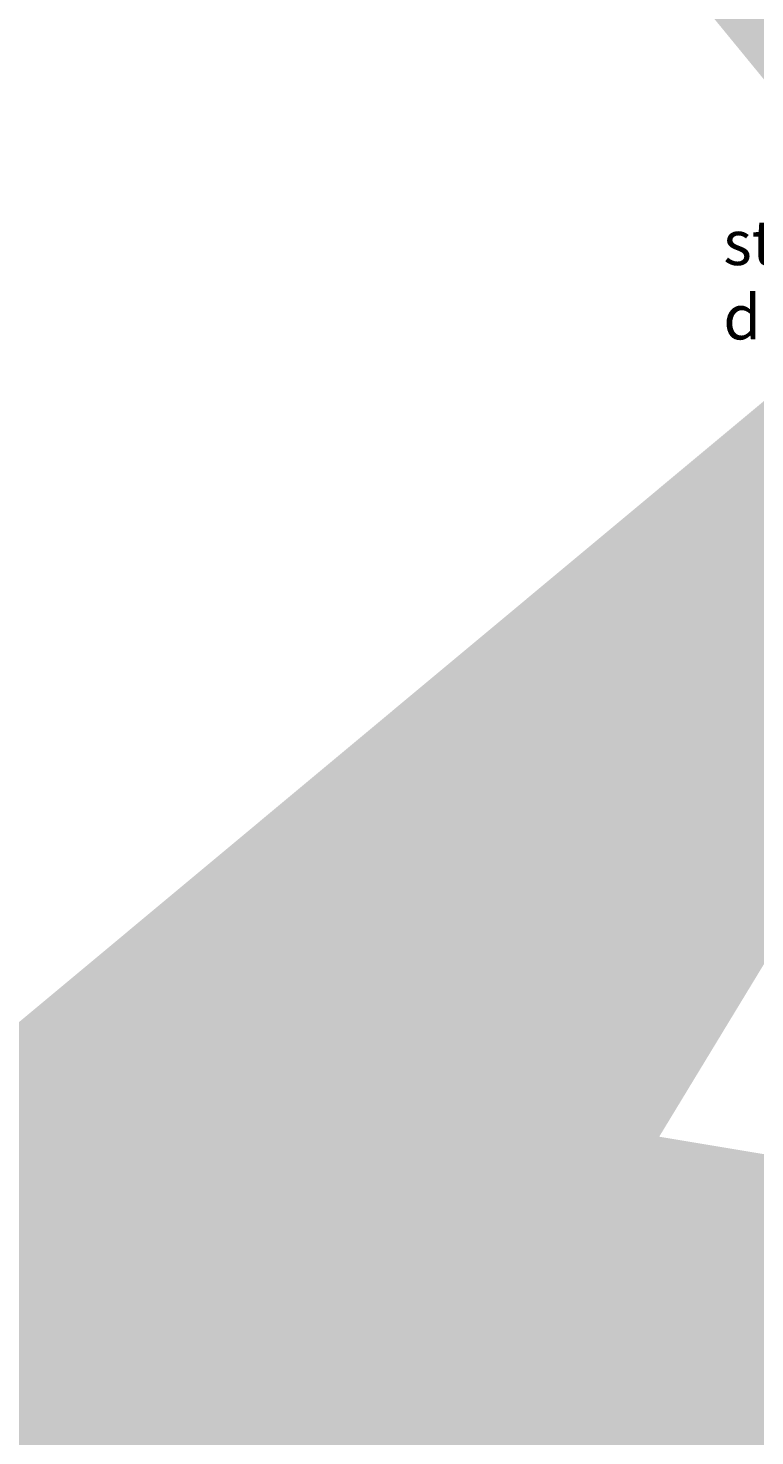
# Model space of a CAD drawing. Units: millimetres. Extents: x -22994 to 29398, y -19990 to 20176.
# Tile 8 of 135: x -44 to 5, y 5 to 99. Entities that reach past the tile are written whole.
import ezdxf

# ---------------------------------------------------------------- set-up
doc = ezdxf.new("R2010")
doc.units = ezdxf.units.MM
doc.header["$MEASUREMENT"] = 0
doc.layers.add('M-ANNO-TEXT', color=7, linetype='Continuous', lineweight=25)
doc.layers.add('M-DIMS', color=2, linetype='Continuous', lineweight=18)
doc.styles.get("Standard").update_dxf_attribs({"font": 'arial.ttf'})
doc.dimstyles.get("Standard").update_dxf_attribs({"dimtxt": 0.18, "dimasz": 10000, "dimexe": 0.18, "dimexo": 0.0625, "dimgap": 0.09, "dimtad": 0, "dimtih": 1, "dimtoh": 1, "dimdec": 0, "dimzin": 0, "dimdsep": 46, "dimtxsty": 'Standard', "dimcen": 0.09, "dimadec": 0, "dimazin": 0, "dimtfac": 1, "dimtdec": 0, "dimtofl": 0, "dimtmove": 0, "dimatfit": 3, "dimfxl": 1, "dimtolj": 1, "dimtzin": 0, "dimlwd": 30, "dimarcsym": 0})

# ---------------------------------------------------------------- blocks, each defined once
blk = doc.blocks.new('*D2')
at = {"layer": 'Defpoints', "color": 0, "transparency": 16777216}
for p in [(6.677, 10.271), (290.852, 10.271), (290.852, -5.079)]:
    blk.add_point(p, dxfattribs=at)
at = {"layer": 'M-DIMS', "color": 0, "lineweight": -2, "transparency": 16777216}
for p, q in [((6.677, 10.209), (6.677, -5.259)), ((290.852, 10.209), (290.852, -5.259))]:
    blk.add_line(p, q, dxfattribs=at)
at = {"layer": 'M-DIMS', "color": 0, "lineweight": 30, "transparency": 16777216}
for p, q in [((-9993.323, -5.079), (-19993.323, -5.079)), ((10290.852, -5.079), (20290.852, -5.079))]:
    blk.add_line(p, q, dxfattribs=at)
at = {"layer": 'M-DIMS', "color": 0, "transparency": 16777216}
for points in [[(-9993.323, 1661.588), (-9993.323, -1671.745), (6.677, -5.079)], [(10290.852, 1661.588), (10290.852, -1671.745), (290.852, -5.079)]]:
    blk.add_solid(points, dxfattribs=at)
at = {"layer": 'M-DIMS', "color": 0, "transparency": 16777216, "insert": (148.765, -5.079), "char_height": 0.18, "attachment_point": 5}
blk.add_mtext('\\A1;284.2', dxfattribs=at)
blk = doc.blocks.new('*D3')
at = {"layer": 'Defpoints', "color": 0, "transparency": 16777216}
for p in [(110.265, 204.165), (110.265, 176.366), (95.833, 127.967)]:
    blk.add_point(p, dxfattribs=at)
at = {"layer": 'M-DIMS', "color": 0, "lineweight": 30, "transparency": 16777216}
for p, q in [((-9904.167, 204.165), (-19904.167, 204.165)), ((10110.265, 204.165), (20110.265, 204.165))]:
    blk.add_line(p, q, dxfattribs=at)
at = {"layer": 'M-DIMS', "color": 0, "lineweight": -2, "transparency": 16777216}
for p, q in [((95.833, 128.03), (95.833, 204.345)), ((110.265, 176.429), (110.265, 204.345))]:
    blk.add_line(p, q, dxfattribs=at)
at = {"layer": 'M-DIMS', "color": 0, "transparency": 16777216}
for points in [[(-9904.167, 1870.832), (-9904.167, -1462.501), (95.833, 204.165)], [(10110.265, 1870.832), (10110.265, -1462.501), (110.265, 204.165)]]:
    blk.add_solid(points, dxfattribs=at)
at = {"layer": 'M-DIMS', "color": 0, "transparency": 16777216, "insert": (103.049, 204.165), "char_height": 0.18, "attachment_point": 5}
blk.add_mtext('\\A1;14.432', dxfattribs=at)
blk = doc.blocks.new('*D4')
at = {"layer": 'Defpoints', "color": 0, "transparency": 16777216}
for p in [(116.265, 204.165), (110.265, 176.366), (116.265, 176.366)]:
    blk.add_point(p, dxfattribs=at)
at = {"layer": 'M-DIMS', "color": 0, "lineweight": 30, "transparency": 16777216}
for p, q in [((-9889.735, 204.165), (-19889.735, 204.165)), ((10116.265, 204.165), (20116.265, 204.165))]:
    blk.add_line(p, q, dxfattribs=at)
at = {"layer": 'M-DIMS', "color": 0, "lineweight": -2, "transparency": 16777216}
for p, q in [((110.265, 176.429), (110.265, 204.345)), ((116.265, 176.429), (116.265, 204.345))]:
    blk.add_line(p, q, dxfattribs=at)
at = {"layer": 'M-DIMS', "color": 0, "transparency": 16777216}
for points in [[(-9889.735, 1870.832), (-9889.735, -1462.501), (110.265, 204.165)], [(10116.265, 1870.832), (10116.265, -1462.501), (116.265, 204.165)]]:
    blk.add_solid(points, dxfattribs=at)
at = {"layer": 'M-DIMS', "color": 0, "transparency": 16777216, "insert": (113.265, 204.165), "char_height": 0.18, "attachment_point": 5}
blk.add_mtext('\\A1;6', dxfattribs=at)
blk = doc.blocks.new('*D5')
at = {"layer": 'Defpoints', "color": 0, "transparency": 16777216}
for p in [(181.265, 204.165), (116.265, 176.366), (181.265, 176.366)]:
    blk.add_point(p, dxfattribs=at)
at = {"layer": 'M-DIMS', "color": 0, "lineweight": 30, "transparency": 16777216}
for p, q in [((-9883.735, 204.165), (-19883.735, 204.165)), ((10181.265, 204.165), (20181.265, 204.165))]:
    blk.add_line(p, q, dxfattribs=at)
at = {"layer": 'M-DIMS', "color": 0, "lineweight": -2, "transparency": 16777216}
for p, q in [((116.265, 176.429), (116.265, 204.345)), ((181.265, 176.429), (181.265, 204.345))]:
    blk.add_line(p, q, dxfattribs=at)
at = {"layer": 'M-DIMS', "color": 0, "transparency": 16777216}
for points in [[(-9883.735, 1870.832), (-9883.735, -1462.501), (116.265, 204.165)], [(10181.265, 1870.832), (10181.265, -1462.501), (181.265, 204.165)]]:
    blk.add_solid(points, dxfattribs=at)
at = {"layer": 'M-DIMS', "color": 0, "transparency": 16777216, "insert": (148.765, 204.165), "char_height": 0.18, "attachment_point": 5}
blk.add_mtext('\\A1;65', dxfattribs=at)
blk = doc.blocks.new('*D6')
at = {"layer": 'Defpoints', "color": 0, "transparency": 16777216}
for p in [(187.265, 204.165), (181.265, 176.366), (187.265, 176.366)]:
    blk.add_point(p, dxfattribs=at)
at = {"layer": 'M-DIMS', "color": 0, "lineweight": 30, "transparency": 16777216}
for p, q in [((-9818.735, 204.165), (-19818.735, 204.165)), ((10187.265, 204.165), (20187.265, 204.165))]:
    blk.add_line(p, q, dxfattribs=at)
at = {"layer": 'M-DIMS', "color": 0, "lineweight": -2, "transparency": 16777216}
for p, q in [((181.265, 176.429), (181.265, 204.345)), ((187.265, 176.429), (187.265, 204.345))]:
    blk.add_line(p, q, dxfattribs=at)
at = {"layer": 'M-DIMS', "color": 0, "transparency": 16777216}
for points in [[(-9818.735, 1870.832), (-9818.735, -1462.501), (181.265, 204.165)], [(10187.265, 1870.832), (10187.265, -1462.501), (187.265, 204.165)]]:
    blk.add_solid(points, dxfattribs=at)
at = {"layer": 'M-DIMS', "color": 0, "transparency": 16777216, "insert": (184.265, 204.165), "char_height": 0.18, "attachment_point": 5}
blk.add_mtext('\\A1;6', dxfattribs=at)
blk = doc.blocks.new('*D7')
at = {"layer": 'Defpoints', "color": 0, "transparency": 16777216}
for p in [(201.697, 204.165), (187.265, 176.366), (201.697, 127.967)]:
    blk.add_point(p, dxfattribs=at)
at = {"layer": 'M-DIMS', "color": 0, "lineweight": 30, "transparency": 16777216}
for p, q in [((-9812.735, 204.165), (-19812.735, 204.165)), ((10201.697, 204.165), (20201.697, 204.165))]:
    blk.add_line(p, q, dxfattribs=at)
at = {"layer": 'M-DIMS', "color": 0, "lineweight": -2, "transparency": 16777216}
for p, q in [((187.265, 176.429), (187.265, 204.345)), ((201.697, 128.03), (201.697, 204.345))]:
    blk.add_line(p, q, dxfattribs=at)
at = {"layer": 'M-DIMS', "color": 0, "transparency": 16777216}
for points in [[(-9812.735, 1870.832), (-9812.735, -1462.501), (187.265, 204.165)], [(10201.697, 1870.832), (10201.697, -1462.501), (201.697, 204.165)]]:
    blk.add_solid(points, dxfattribs=at)
at = {"layer": 'M-DIMS', "color": 0, "transparency": 16777216, "insert": (194.481, 204.165), "char_height": 0.18, "attachment_point": 5}
blk.add_mtext('\\A1;14.432', dxfattribs=at)
blk = doc.blocks.new('*D8')
at = {"layer": 'Defpoints', "color": 0, "transparency": 16777216}
for p in [(227.648, 204.165), (227.648, 146.73), (201.697, 127.967)]:
    blk.add_point(p, dxfattribs=at)
at = {"layer": 'M-DIMS', "color": 0, "lineweight": 30, "transparency": 16777216}
for p, q in [((-9798.303, 204.165), (-19798.303, 204.165)), ((10227.648, 204.165), (20227.648, 204.165))]:
    blk.add_line(p, q, dxfattribs=at)
at = {"layer": 'M-DIMS', "color": 0, "lineweight": -2, "transparency": 16777216}
for p, q in [((201.697, 128.03), (201.697, 204.345)), ((227.648, 146.792), (227.648, 204.345))]:
    blk.add_line(p, q, dxfattribs=at)
at = {"layer": 'M-DIMS', "color": 0, "transparency": 16777216}
for points in [[(-9798.303, 1870.832), (-9798.303, -1462.501), (201.697, 204.165)], [(10227.648, 1870.832), (10227.648, -1462.501), (227.648, 204.165)]]:
    blk.add_solid(points, dxfattribs=at)
at = {"layer": 'M-DIMS', "color": 0, "transparency": 16777216, "insert": (214.673, 204.165), "char_height": 0.18, "attachment_point": 5}
blk.add_mtext('\\A1;25.95', dxfattribs=at)
blk = doc.blocks.new('*D9')
at = {"layer": 'Defpoints', "color": 0, "transparency": 16777216}
for p in [(187.265, 176.366), (306.202, 176.366), (290.852, 10.271)]:
    blk.add_point(p, dxfattribs=at)
at = {"layer": 'M-DIMS', "color": 0, "lineweight": 30, "transparency": 16777216}
for p, q in [((306.202, 10176.366), (306.202, 20176.366)), ((306.202, -9989.729), (306.202, -19989.729))]:
    blk.add_line(p, q, dxfattribs=at)
at = {"layer": 'M-DIMS', "color": 0, "lineweight": -2, "transparency": 16777216}
for p, q in [((187.327, 176.366), (306.382, 176.366)), ((290.915, 10.271), (306.382, 10.271))]:
    blk.add_line(p, q, dxfattribs=at)
at = {"layer": 'M-DIMS', "color": 0, "transparency": 16777216}
for points in [[(-1360.465, 10176.366), (1972.869, 10176.366), (306.202, 176.366)], [(-1360.465, -9989.729), (1972.869, -9989.729), (306.202, 10.271)]]:
    blk.add_solid(points, dxfattribs=at)
at = {"layer": 'M-DIMS', "color": 0, "transparency": 16777216, "insert": (306.202, 93.319), "char_height": 0.18, "attachment_point": 5}
blk.add_mtext('\\A1;166.1', dxfattribs=at)
blk = doc.blocks.new('*D10')
at = {"layer": 'Defpoints', "color": 0, "transparency": 16777216}
for p in [(125.65, 136.071), (133.346, 136.071), (133.346, -5.079)]:
    blk.add_point(p, dxfattribs=at)
at = {"layer": 'M-DIMS', "color": 0, "lineweight": -2, "transparency": 16777216}
for p, q in [((125.65, 136.009), (125.65, -5.259)), ((133.346, 136.009), (133.346, -5.259))]:
    blk.add_line(p, q, dxfattribs=at)
at = {"layer": 'M-DIMS', "color": 0, "lineweight": 30, "transparency": 16777216}
for p, q in [((-9874.35, -5.079), (-19874.35, -5.079)), ((10133.346, -5.079), (20133.346, -5.079))]:
    blk.add_line(p, q, dxfattribs=at)
at = {"layer": 'M-DIMS', "color": 0, "transparency": 16777216}
for points in [[(-9874.35, 1661.588), (-9874.35, -1671.745), (125.65, -5.079)], [(10133.346, 1661.588), (10133.346, -1671.745), (133.346, -5.079)]]:
    blk.add_solid(points, dxfattribs=at)
at = {"layer": 'M-DIMS', "color": 0, "transparency": 16777216, "insert": (129.498, -5.079), "char_height": 0.18, "attachment_point": 5}
blk.add_mtext('\\A1;7.696', dxfattribs=at)
blk = doc.blocks.new('*D11')
at = {"layer": 'Defpoints', "color": 0, "transparency": 16777216}
for p in [(133.346, 136.071), (135.65, 136.071), (135.65, -5.079)]:
    blk.add_point(p, dxfattribs=at)
at = {"layer": 'M-DIMS', "color": 0, "lineweight": -2, "transparency": 16777216}
for p, q in [((133.346, 136.009), (133.346, -5.259)), ((135.65, 136.009), (135.65, -5.259))]:
    blk.add_line(p, q, dxfattribs=at)
at = {"layer": 'M-DIMS', "color": 0, "lineweight": 30, "transparency": 16777216}
for p, q in [((-9866.654, -5.079), (-19866.654, -5.079)), ((10135.65, -5.079), (20135.65, -5.079))]:
    blk.add_line(p, q, dxfattribs=at)
at = {"layer": 'M-DIMS', "color": 0, "transparency": 16777216}
for points in [[(-9866.654, 1661.588), (-9866.654, -1671.745), (133.346, -5.079)], [(10135.65, 1661.588), (10135.65, -1671.745), (135.65, -5.079)]]:
    blk.add_solid(points, dxfattribs=at)
at = {"layer": 'M-DIMS', "color": 0, "transparency": 16777216, "insert": (134.498, -5.079), "char_height": 0.18, "attachment_point": 5}
blk.add_mtext('\\A1;2.304', dxfattribs=at)
blk = doc.blocks.new('*D12')
at = {"layer": 'Defpoints', "color": 0, "transparency": 16777216}
for p in [(135.65, 136.071), (145.65, 136.071), (145.65, -5.079)]:
    blk.add_point(p, dxfattribs=at)
at = {"layer": 'M-DIMS', "color": 0, "lineweight": -2, "transparency": 16777216}
for p, q in [((135.65, 136.009), (135.65, -5.259)), ((145.65, 136.009), (145.65, -5.259))]:
    blk.add_line(p, q, dxfattribs=at)
at = {"layer": 'M-DIMS', "color": 0, "lineweight": 30, "transparency": 16777216}
for p, q in [((-9864.35, -5.079), (-19864.35, -5.079)), ((10145.65, -5.079), (20145.65, -5.079))]:
    blk.add_line(p, q, dxfattribs=at)
at = {"layer": 'M-DIMS', "color": 0, "transparency": 16777216}
for points in [[(-9864.35, 1661.588), (-9864.35, -1671.745), (135.65, -5.079)], [(10145.65, 1661.588), (10145.65, -1671.745), (145.65, -5.079)]]:
    blk.add_solid(points, dxfattribs=at)
at = {"layer": 'M-DIMS', "color": 0, "transparency": 16777216, "insert": (140.65, -5.079), "char_height": 0.18, "attachment_point": 5}
blk.add_mtext('\\A1;10', dxfattribs=at)
blk = doc.blocks.new('*D13')
at = {"layer": 'Defpoints', "color": 0, "transparency": 16777216}
for p in [(145.65, 136.071), (155.65, 136.071), (155.65, -5.079)]:
    blk.add_point(p, dxfattribs=at)
at = {"layer": 'M-DIMS', "color": 0, "lineweight": -2, "transparency": 16777216}
for p, q in [((145.65, 136.009), (145.65, -5.259)), ((155.65, 136.009), (155.65, -5.259))]:
    blk.add_line(p, q, dxfattribs=at)
at = {"layer": 'M-DIMS', "color": 0, "lineweight": 30, "transparency": 16777216}
for p, q in [((-9854.35, -5.079), (-19854.35, -5.079)), ((10155.65, -5.079), (20155.65, -5.079))]:
    blk.add_line(p, q, dxfattribs=at)
at = {"layer": 'M-DIMS', "color": 0, "transparency": 16777216}
for points in [[(-9854.35, 1661.588), (-9854.35, -1671.745), (145.65, -5.079)], [(10155.65, 1661.588), (10155.65, -1671.745), (155.65, -5.079)]]:
    blk.add_solid(points, dxfattribs=at)
at = {"layer": 'M-DIMS', "color": 0, "transparency": 16777216, "insert": (150.65, -5.079), "char_height": 0.18, "attachment_point": 5}
blk.add_mtext('\\A1;10', dxfattribs=at)
blk = doc.blocks.new('*D14')
at = {"layer": 'Defpoints', "color": 0, "transparency": 16777216}
for p in [(155.65, 136.071), (165.65, 136.071), (165.65, -5.079)]:
    blk.add_point(p, dxfattribs=at)
at = {"layer": 'M-DIMS', "color": 0, "lineweight": -2, "transparency": 16777216}
for p, q in [((155.65, 136.009), (155.65, -5.259)), ((165.65, 136.009), (165.65, -5.259))]:
    blk.add_line(p, q, dxfattribs=at)
at = {"layer": 'M-DIMS', "color": 0, "lineweight": 30, "transparency": 16777216}
for p, q in [((-9844.35, -5.079), (-19844.35, -5.079)), ((10165.65, -5.079), (20165.65, -5.079))]:
    blk.add_line(p, q, dxfattribs=at)
at = {"layer": 'M-DIMS', "color": 0, "transparency": 16777216}
for points in [[(-9844.35, 1661.588), (-9844.35, -1671.745), (155.65, -5.079)], [(10165.65, 1661.588), (10165.65, -1671.745), (165.65, -5.079)]]:
    blk.add_solid(points, dxfattribs=at)
at = {"layer": 'M-DIMS', "color": 0, "transparency": 16777216, "insert": (160.65, -5.079), "char_height": 0.18, "attachment_point": 5}
blk.add_mtext('\\A1;10', dxfattribs=at)
blk = doc.blocks.new('*D15')
at = {"layer": 'Defpoints', "color": 0, "transparency": 16777216}
for p in [(173.346, 154.788), (173.346, 136.071), (306.202, 136.071)]:
    blk.add_point(p, dxfattribs=at)
at = {"layer": 'M-DIMS', "color": 0, "lineweight": 30, "transparency": 16777216}
for p, q in [((306.202, 10154.788), (306.202, 20154.788)), ((306.202, -9863.929), (306.202, -19863.929))]:
    blk.add_line(p, q, dxfattribs=at)
at = {"layer": 'M-DIMS', "color": 0, "lineweight": -2, "transparency": 16777216}
for p, q in [((173.408, 154.788), (306.382, 154.788)), ((173.408, 136.071), (306.382, 136.071))]:
    blk.add_line(p, q, dxfattribs=at)
at = {"layer": 'M-DIMS', "color": 0, "transparency": 16777216}
for points in [[(-1360.465, 10154.788), (1972.869, 10154.788), (306.202, 154.788)], [(-1360.465, -9863.929), (1972.869, -9863.929), (306.202, 136.071)]]:
    blk.add_solid(points, dxfattribs=at)
at = {"layer": 'M-DIMS', "color": 0, "transparency": 16777216, "insert": (306.202, 145.43), "char_height": 0.18, "attachment_point": 5}
blk.add_mtext('\\A1;18.717', dxfattribs=at)
blk = doc.blocks.new('*D16')
at = {"layer": 'Defpoints', "color": 0, "transparency": 16777216}
for p in [(120.17, 204.165), (110.466, 48.035), (120.17, 48.035)]:
    blk.add_point(p, dxfattribs=at)
at = {"layer": 'M-DIMS', "color": 0, "lineweight": 30, "transparency": 16777216}
for p, q in [((-9889.534, 204.165), (-19889.534, 204.165)), ((10120.17, 204.165), (20120.17, 204.165))]:
    blk.add_line(p, q, dxfattribs=at)
at = {"layer": 'M-DIMS', "color": 0, "lineweight": -2, "transparency": 16777216}
for p, q in [((110.466, 48.097), (110.466, 204.345)), ((120.17, 48.097), (120.17, 204.345))]:
    blk.add_line(p, q, dxfattribs=at)
at = {"layer": 'M-DIMS', "color": 0, "transparency": 16777216}
for points in [[(-9889.534, 1870.832), (-9889.534, -1462.501), (110.466, 204.165)], [(10120.17, 1870.832), (10120.17, -1462.501), (120.17, 204.165)]]:
    blk.add_solid(points, dxfattribs=at)
at = {"layer": 'M-DIMS', "color": 0, "transparency": 16777216, "insert": (115.318, 204.165), "char_height": 0.18, "attachment_point": 5}
blk.add_mtext('\\A1;9.704', dxfattribs=at)
blk = doc.blocks.new('*D17')
at = {"layer": 'Defpoints', "color": 0, "transparency": 16777216}
for p in [(126.17, 204.165), (120.17, 48.035), (126.17, 48.035)]:
    blk.add_point(p, dxfattribs=at)
at = {"layer": 'M-DIMS', "color": 0, "lineweight": 30, "transparency": 16777216}
for p, q in [((-9879.83, 204.165), (-19879.83, 204.165)), ((10126.17, 204.165), (20126.17, 204.165))]:
    blk.add_line(p, q, dxfattribs=at)
at = {"layer": 'M-DIMS', "color": 0, "lineweight": -2, "transparency": 16777216}
for p, q in [((120.17, 48.097), (120.17, 204.345)), ((126.17, 48.097), (126.17, 204.345))]:
    blk.add_line(p, q, dxfattribs=at)
at = {"layer": 'M-DIMS', "color": 0, "transparency": 16777216}
for points in [[(-9879.83, 1870.832), (-9879.83, -1462.501), (120.17, 204.165)], [(10126.17, 1870.832), (10126.17, -1462.501), (126.17, 204.165)]]:
    blk.add_solid(points, dxfattribs=at)
at = {"layer": 'M-DIMS', "color": 0, "transparency": 16777216, "insert": (123.17, 204.165), "char_height": 0.18, "attachment_point": 5}
blk.add_mtext('\\A1;6', dxfattribs=at)
blk = doc.blocks.new('*D18')
at = {"layer": 'Defpoints', "color": 0, "transparency": 16777216}
for p in [(132.17, 204.165), (126.17, 48.035), (132.17, 48.035)]:
    blk.add_point(p, dxfattribs=at)
at = {"layer": 'M-DIMS', "color": 0, "lineweight": 30, "transparency": 16777216}
for p, q in [((-9873.83, 204.165), (-19873.83, 204.165)), ((10132.17, 204.165), (20132.17, 204.165))]:
    blk.add_line(p, q, dxfattribs=at)
at = {"layer": 'M-DIMS', "color": 0, "lineweight": -2, "transparency": 16777216}
for p, q in [((126.17, 48.097), (126.17, 204.345)), ((132.17, 48.097), (132.17, 204.345))]:
    blk.add_line(p, q, dxfattribs=at)
at = {"layer": 'M-DIMS', "color": 0, "transparency": 16777216}
for points in [[(-9873.83, 1870.832), (-9873.83, -1462.501), (126.17, 204.165)], [(10132.17, 1870.832), (10132.17, -1462.501), (132.17, 204.165)]]:
    blk.add_solid(points, dxfattribs=at)
at = {"layer": 'M-DIMS', "color": 0, "transparency": 16777216, "insert": (129.17, 204.165), "char_height": 0.18, "attachment_point": 5}
blk.add_mtext('\\A1;6', dxfattribs=at)
blk = doc.blocks.new('*D19')
at = {"layer": 'Defpoints', "color": 0, "transparency": 16777216}
for p in [(138.17, 204.165), (132.17, 48.035), (138.17, 48.035)]:
    blk.add_point(p, dxfattribs=at)
at = {"layer": 'M-DIMS', "color": 0, "lineweight": 30, "transparency": 16777216}
for p, q in [((-9867.83, 204.165), (-19867.83, 204.165)), ((10138.17, 204.165), (20138.17, 204.165))]:
    blk.add_line(p, q, dxfattribs=at)
at = {"layer": 'M-DIMS', "color": 0, "lineweight": -2, "transparency": 16777216}
for p, q in [((132.17, 48.097), (132.17, 204.345)), ((138.17, 48.097), (138.17, 204.345))]:
    blk.add_line(p, q, dxfattribs=at)
at = {"layer": 'M-DIMS', "color": 0, "transparency": 16777216}
for points in [[(-9867.83, 1870.832), (-9867.83, -1462.501), (132.17, 204.165)], [(10138.17, 1870.832), (10138.17, -1462.501), (138.17, 204.165)]]:
    blk.add_solid(points, dxfattribs=at)
at = {"layer": 'M-DIMS', "color": 0, "transparency": 16777216, "insert": (135.17, 204.165), "char_height": 0.18, "attachment_point": 5}
blk.add_mtext('\\A1;6', dxfattribs=at)
blk = doc.blocks.new('*D20')
at = {"layer": 'Defpoints', "color": 0, "transparency": 16777216}
for p in [(144.17, 204.165), (138.17, 48.035), (144.17, 48.035)]:
    blk.add_point(p, dxfattribs=at)
at = {"layer": 'M-DIMS', "color": 0, "lineweight": 30, "transparency": 16777216}
for p, q in [((-9861.83, 204.165), (-19861.83, 204.165)), ((10144.17, 204.165), (20144.17, 204.165))]:
    blk.add_line(p, q, dxfattribs=at)
at = {"layer": 'M-DIMS', "color": 0, "lineweight": -2, "transparency": 16777216}
for p, q in [((138.17, 48.097), (138.17, 204.345)), ((144.17, 48.097), (144.17, 204.345))]:
    blk.add_line(p, q, dxfattribs=at)
at = {"layer": 'M-DIMS', "color": 0, "transparency": 16777216}
for points in [[(-9861.83, 1870.832), (-9861.83, -1462.501), (138.17, 204.165)], [(10144.17, 1870.832), (10144.17, -1462.501), (144.17, 204.165)]]:
    blk.add_solid(points, dxfattribs=at)
at = {"layer": 'M-DIMS', "color": 0, "transparency": 16777216, "insert": (141.17, 204.165), "char_height": 0.18, "attachment_point": 5}
blk.add_mtext('\\A1;6', dxfattribs=at)
blk = doc.blocks.new('*D21')
at = {"layer": 'Defpoints', "color": 0, "transparency": 16777216}
for p in [(149.116, 204.165), (144.17, 48.035), (149.116, 48.035)]:
    blk.add_point(p, dxfattribs=at)
at = {"layer": 'M-DIMS', "color": 0, "lineweight": 30, "transparency": 16777216}
for p, q in [((-9855.83, 204.165), (-19855.83, 204.165)), ((10149.116, 204.165), (20149.116, 204.165))]:
    blk.add_line(p, q, dxfattribs=at)
at = {"layer": 'M-DIMS', "color": 0, "lineweight": -2, "transparency": 16777216}
for p, q in [((144.17, 48.097), (144.17, 204.345)), ((149.116, 48.097), (149.116, 204.345))]:
    blk.add_line(p, q, dxfattribs=at)
at = {"layer": 'M-DIMS', "color": 0, "transparency": 16777216}
for points in [[(-9855.83, 1870.832), (-9855.83, -1462.501), (144.17, 204.165)], [(10149.116, 1870.832), (10149.116, -1462.501), (149.116, 204.165)]]:
    blk.add_solid(points, dxfattribs=at)
at = {"layer": 'M-DIMS', "color": 0, "transparency": 16777216, "insert": (146.643, 204.165), "char_height": 0.18, "attachment_point": 5}
blk.add_mtext('\\A1;4.945', dxfattribs=at)
blk = doc.blocks.new('*D22')
at = {"layer": 'Defpoints', "color": 0, "transparency": 16777216}
for p in [(149.116, 30.99), (155.116, 30.99), (155.116, -5.079)]:
    blk.add_point(p, dxfattribs=at)
at = {"layer": 'M-DIMS', "color": 0, "lineweight": -2, "transparency": 16777216}
for p, q in [((149.116, 30.927), (149.116, -5.259)), ((155.116, 30.927), (155.116, -5.259))]:
    blk.add_line(p, q, dxfattribs=at)
at = {"layer": 'M-DIMS', "color": 0, "lineweight": 30, "transparency": 16777216}
for p, q in [((-9850.884, -5.079), (-19850.884, -5.079)), ((10155.116, -5.079), (20155.116, -5.079))]:
    blk.add_line(p, q, dxfattribs=at)
at = {"layer": 'M-DIMS', "color": 0, "transparency": 16777216}
for points in [[(-9850.884, 1661.588), (-9850.884, -1671.745), (149.116, -5.079)], [(10155.116, 1661.588), (10155.116, -1671.745), (155.116, -5.079)]]:
    blk.add_solid(points, dxfattribs=at)
at = {"layer": 'M-DIMS', "color": 0, "transparency": 16777216, "insert": (152.116, -5.079), "char_height": 0.18, "attachment_point": 5}
blk.add_mtext('\\A1;6', dxfattribs=at)
blk = doc.blocks.new('*D23')
at = {"layer": 'Defpoints', "color": 0, "transparency": 16777216}
for p in [(155.116, 30.99), (161.116, 30.99), (161.116, -5.079)]:
    blk.add_point(p, dxfattribs=at)
at = {"layer": 'M-DIMS', "color": 0, "lineweight": -2, "transparency": 16777216}
for p, q in [((155.116, 30.927), (155.116, -5.259)), ((161.116, 30.927), (161.116, -5.259))]:
    blk.add_line(p, q, dxfattribs=at)
at = {"layer": 'M-DIMS', "color": 0, "lineweight": 30, "transparency": 16777216}
for p, q in [((-9844.884, -5.079), (-19844.884, -5.079)), ((10161.116, -5.079), (20161.116, -5.079))]:
    blk.add_line(p, q, dxfattribs=at)
at = {"layer": 'M-DIMS', "color": 0, "transparency": 16777216}
for points in [[(-9844.884, 1661.588), (-9844.884, -1671.745), (155.116, -5.079)], [(10161.116, 1661.588), (10161.116, -1671.745), (161.116, -5.079)]]:
    blk.add_solid(points, dxfattribs=at)
at = {"layer": 'M-DIMS', "color": 0, "transparency": 16777216, "insert": (158.116, -5.079), "char_height": 0.18, "attachment_point": 5}
blk.add_mtext('\\A1;6', dxfattribs=at)
blk = doc.blocks.new('*D24')
at = {"layer": 'Defpoints', "color": 0, "transparency": 16777216}
for p in [(161.116, 30.99), (166.439, 30.99), (166.439, -5.079)]:
    blk.add_point(p, dxfattribs=at)
at = {"layer": 'M-DIMS', "color": 0, "lineweight": -2, "transparency": 16777216}
for p, q in [((161.116, 30.927), (161.116, -5.259)), ((166.439, 30.927), (166.439, -5.259))]:
    blk.add_line(p, q, dxfattribs=at)
at = {"layer": 'M-DIMS', "color": 0, "lineweight": 30, "transparency": 16777216}
for p, q in [((-9838.884, -5.079), (-19838.884, -5.079)), ((10166.439, -5.079), (20166.439, -5.079))]:
    blk.add_line(p, q, dxfattribs=at)
at = {"layer": 'M-DIMS', "color": 0, "transparency": 16777216}
for points in [[(-9838.884, 1661.588), (-9838.884, -1671.745), (161.116, -5.079)], [(10166.439, 1661.588), (10166.439, -1671.745), (166.439, -5.079)]]:
    blk.add_solid(points, dxfattribs=at)
at = {"layer": 'M-DIMS', "color": 0, "transparency": 16777216, "insert": (163.777, -5.079), "char_height": 0.18, "attachment_point": 5}
blk.add_mtext('\\A1;5.323', dxfattribs=at)
blk = doc.blocks.new('*D25')
at = {"layer": 'Defpoints', "color": 0, "transparency": 16777216}
for p in [(166.439, 30.99), (172.439, 30.99), (172.439, -5.079)]:
    blk.add_point(p, dxfattribs=at)
at = {"layer": 'M-DIMS', "color": 0, "lineweight": -2, "transparency": 16777216}
for p, q in [((166.439, 30.927), (166.439, -5.259)), ((172.439, 30.927), (172.439, -5.259))]:
    blk.add_line(p, q, dxfattribs=at)
at = {"layer": 'M-DIMS', "color": 0, "lineweight": 30, "transparency": 16777216}
for p, q in [((-9833.561, -5.079), (-19833.561, -5.079)), ((10172.439, -5.079), (20172.439, -5.079))]:
    blk.add_line(p, q, dxfattribs=at)
at = {"layer": 'M-DIMS', "color": 0, "transparency": 16777216}
for points in [[(-9833.561, 1661.588), (-9833.561, -1671.745), (166.439, -5.079)], [(10172.439, 1661.588), (10172.439, -1671.745), (172.439, -5.079)]]:
    blk.add_solid(points, dxfattribs=at)
at = {"layer": 'M-DIMS', "color": 0, "transparency": 16777216, "insert": (169.439, -5.079), "char_height": 0.18, "attachment_point": 5}
blk.add_mtext('\\A1;6', dxfattribs=at)
blk = doc.blocks.new('*D26')
at = {"layer": 'Defpoints', "color": 0, "transparency": 16777216}
for p in [(172.439, 30.99), (178.439, 30.99), (178.439, -5.079)]:
    blk.add_point(p, dxfattribs=at)
at = {"layer": 'M-DIMS', "color": 0, "lineweight": -2, "transparency": 16777216}
for p, q in [((172.439, 30.927), (172.439, -5.259)), ((178.439, 30.927), (178.439, -5.259))]:
    blk.add_line(p, q, dxfattribs=at)
at = {"layer": 'M-DIMS', "color": 0, "lineweight": 30, "transparency": 16777216}
for p, q in [((-9827.561, -5.079), (-19827.561, -5.079)), ((10178.439, -5.079), (20178.439, -5.079))]:
    blk.add_line(p, q, dxfattribs=at)
at = {"layer": 'M-DIMS', "color": 0, "transparency": 16777216}
for points in [[(-9827.561, 1661.588), (-9827.561, -1671.745), (172.439, -5.079)], [(10178.439, 1661.588), (10178.439, -1671.745), (178.439, -5.079)]]:
    blk.add_solid(points, dxfattribs=at)
at = {"layer": 'M-DIMS', "color": 0, "transparency": 16777216, "insert": (175.439, -5.079), "char_height": 0.18, "attachment_point": 5}
blk.add_mtext('\\A1;6', dxfattribs=at)
blk = doc.blocks.new('*D27')
at = {"layer": 'Defpoints', "color": 0, "transparency": 16777216}
for p in [(178.439, 30.99), (188.117, 30.99), (188.117, -5.079)]:
    blk.add_point(p, dxfattribs=at)
at = {"layer": 'M-DIMS', "color": 0, "lineweight": -2, "transparency": 16777216}
for p, q in [((178.439, 30.927), (178.439, -5.259)), ((188.117, 30.927), (188.117, -5.259))]:
    blk.add_line(p, q, dxfattribs=at)
at = {"layer": 'M-DIMS', "color": 0, "lineweight": 30, "transparency": 16777216}
for p, q in [((-9821.561, -5.079), (-19821.561, -5.079)), ((10188.117, -5.079), (20188.117, -5.079))]:
    blk.add_line(p, q, dxfattribs=at)
at = {"layer": 'M-DIMS', "color": 0, "transparency": 16777216}
for points in [[(-9821.561, 1661.588), (-9821.561, -1671.745), (178.439, -5.079)], [(10188.117, 1661.588), (10188.117, -1671.745), (188.117, -5.079)]]:
    blk.add_solid(points, dxfattribs=at)
at = {"layer": 'M-DIMS', "color": 0, "transparency": 16777216, "insert": (183.278, -5.079), "char_height": 0.18, "attachment_point": 5}
blk.add_mtext('\\A1;9.679', dxfattribs=at)
blk = doc.blocks.new('*D28')
at = {"layer": 'Defpoints', "color": 0, "transparency": 16777216}
for p in [(188.117, 48.035), (306.202, 48.035), (188.117, 30.99)]:
    blk.add_point(p, dxfattribs=at)
at = {"layer": 'M-DIMS', "color": 0, "lineweight": 30, "transparency": 16777216}
for p, q in [((306.202, 10048.035), (306.202, 20048.035)), ((306.202, -9969.01), (306.202, -19969.01))]:
    blk.add_line(p, q, dxfattribs=at)
at = {"layer": 'M-DIMS', "color": 0, "lineweight": -2, "transparency": 16777216}
for p, q in [((188.18, 48.035), (306.382, 48.035)), ((188.18, 30.99), (306.382, 30.99))]:
    blk.add_line(p, q, dxfattribs=at)
at = {"layer": 'M-DIMS', "color": 0, "transparency": 16777216}
for points in [[(-1360.465, 10048.035), (1972.869, 10048.035), (306.202, 48.035)], [(-1360.465, -9969.01), (1972.869, -9969.01), (306.202, 30.99)]]:
    blk.add_solid(points, dxfattribs=at)
at = {"layer": 'M-DIMS', "color": 0, "transparency": 16777216, "insert": (306.202, 39.512), "char_height": 0.18, "attachment_point": 5}
blk.add_mtext('\\A1;17.045', dxfattribs=at)
blk = doc.blocks.new('*D32')
at = {"layer": 'Defpoints', "color": 0, "transparency": 16777216}
for p in [(57.164, 118.614), (52.413, 113.093)]:
    blk.add_point(p, dxfattribs=at)
at = {"layer": 'M-DIMS', "color": 0, "lineweight": -2, "transparency": 16777216}
for p, q in [((57.074, 118.614), (57.254, 118.614)), ((57.164, 118.524), (57.164, 118.704))]:
    blk.add_line(p, q, dxfattribs=at)
at = {"layer": 'M-DIMS', "color": 0, "lineweight": 30, "transparency": 16777216}
for p, q in [((-12992.534, -15047.031), (-6470.06, -7466.969)), ((-22992.534, -15047.031), (-12992.534, -15047.031))]:
    blk.add_line(p, q, dxfattribs=at)
at = {"layer": 'M-DIMS', "color": 0, "transparency": 16777216}
blk.add_solid([(-7733.404, -6379.89), (-5206.717, -8554.048), (52.413, 113.093)], dxfattribs=at)
at = {"layer": 'M-DIMS', "color": 0, "transparency": 16777216, "insert": (-22993.208, -15047.031), "char_height": 0.18, "attachment_point": 5}
blk.add_mtext('\\A1;2X R7.284', dxfattribs=at)
blk = doc.blocks.new('*D35')
at = {"layer": 'Defpoints', "color": 0, "transparency": 16777216}
for p in [(21.093, 77.393), (21.84, 76.092)]:
    blk.add_point(p, dxfattribs=at)
at = {"layer": 'M-DIMS', "color": 0, "lineweight": 30, "transparency": 16777216}
for p, q in [((-19938.013, 17421.447), (-9938.013, 17421.447)), ((-9938.013, 17421.447), (-4958.46, 8749.42))]:
    blk.add_line(p, q, dxfattribs=at)
at = {"layer": 'M-DIMS', "color": 0, "lineweight": -2, "transparency": 16777216}
for p, q in [((21.75, 76.092), (21.93, 76.092)), ((21.84, 76.002), (21.84, 76.182))]:
    blk.add_line(p, q, dxfattribs=at)
at = {"layer": 'M-DIMS', "color": 0, "transparency": 16777216}
blk.add_solid([(-3513.122, 9579.345), (-6403.798, 7919.494), (21.093, 77.393)], dxfattribs=at)
at = {"layer": 'M-DIMS', "color": 0, "transparency": 16777216, "insert": (-19938.354, 17421.447), "char_height": 0.18, "attachment_point": 5}
blk.add_mtext('\\A1;R1.5', dxfattribs=at)
blk = doc.blocks.new('*D36')
at = {"layer": 'Defpoints', "color": 0, "transparency": 16777216}
for p in [(46.39, 31.303), (46.387, 26.593)]:
    blk.add_point(p, dxfattribs=at)
at = {"layer": 'M-DIMS', "color": 0, "lineweight": 30, "transparency": 16777216}
for p, q in [((57.15, 20031.301), (51.77, 10031.302)), ((10057.15, 20031.301), (57.15, 20031.301))]:
    blk.add_line(p, q, dxfattribs=at)
at = {"layer": 'M-DIMS', "color": 0, "lineweight": -2, "transparency": 16777216}
for p, q in [((46.299, 28.948), (46.479, 28.948)), ((46.389, 28.858), (46.389, 29.038))]:
    blk.add_line(p, q, dxfattribs=at)
at = {"layer": 'M-DIMS', "color": 0, "transparency": 16777216}
blk.add_solid([(-1614.896, 10032.199), (1718.436, 10030.405), (46.39, 31.303)], dxfattribs=at)
at = {"layer": 'M-DIMS', "color": 0, "transparency": 16777216, "insert": (10057.554, 20031.301), "char_height": 0.18, "attachment_point": 5}
blk.add_mtext('\\A1;∅4.71', dxfattribs=at)

msp = doc.modelspace()

# ---------------------------------------------------------------- texts
at = {"layer": 'M-ANNO-TEXT', "insert": (3.1749, 86.4503), "char_height": 3, "attachment_point": 1}
msp.add_mtext_dynamic_manual_height_columns('steam separating\\Pdrum', width=37.883315, gutter_width=1, heights=[0], dxfattribs=at)

# ---------------------------------------------------------------- dimensions: what is measured, and where the dimension line sits
at = {"layer": 'M-DIMS'}
for base, p1, p2, override, picture, middle in [((306.202, 176.3662), (290.852, 10.2713), (187.2647, 176.3662), {"dimdec": 1, "dimlfac": 1, "dimrnd": 0, "dimzin": 0, "dimdsep": 46, "dimlunit": 2}, '*D9', (306.202, 93.3187)), ((306.202, 136.0713), (173.3459, 154.788), (173.3459, 136.0713), {"dimdec": 3, "dimlfac": 1, "dimrnd": 0, "dimzin": 0, "dimdsep": 46, "dimlunit": 2}, '*D15', (306.202, 145.4297)), ((306.202, 48.0349), (188.1175, 30.9895), (188.1175, 48.0349), {"dimdec": 3, "dimlfac": 1, "dimrnd": 0, "dimzin": 0, "dimdsep": 46, "dimlunit": 2}, '*D28', (306.202, 39.5122))]:
    dim = msp.add_linear_dim(base=base, p1=p1, p2=p2, angle=90, dimstyle='Standard', override=override, dxfattribs=at)
    dim.commit()
    dim.dimension.update_dxf_attribs({"geometry": picture, "text_midpoint": middle})
dim = msp.add_diameter_dim_2p(p1=(46.3875, 26.5934), p2=(46.39, 31.3035), dimstyle='Standard', override={"dimdec": 2, "dimlfac": 1, "dimrnd": 0, "dimzin": 0, "dimdsep": 46, "dimlunit": 2}, dxfattribs=at)
dim.commit()
dim.dimension.update_dxf_attribs({"geometry": '*D36', "text_midpoint": (10057.5542, 20031.3006), "dimtype": 163})
dim = msp.add_radius_dim(center=(21.8402, 76.0922), mpoint=(21.0933, 77.393), dimstyle='Standard', override={"dimdec": 1, "dimlfac": 1, "dimrnd": 0, "dimzin": 0, "dimdsep": 46, "dimlunit": 2}, dxfattribs=at)
dim.commit()
dim.dimension.update_dxf_attribs({"geometry": '*D35', "text_midpoint": (-19938.3541, 17421.4466)})
for base, p1, p2, override, picture, middle in [((110.2647, 204.1654), (95.8327, 127.967), (110.2647, 176.3662), {"dimdec": 3, "dimlfac": 1, "dimrnd": 0, "dimzin": 0, "dimdsep": 46, "dimlunit": 2}, '*D3', (103.0487, 204.1654)), ((116.2647, 204.1654), (110.2647, 176.3662), (116.2647, 176.3662), {"dimdec": 0, "dimlfac": 1, "dimrnd": 0, "dimzin": 0, "dimdsep": 46, "dimlunit": 2}, '*D4', (113.2647, 204.1654)), ((120.1702, 204.1654), (110.4658, 48.0349), (120.1702, 48.0349), {"dimdec": 3, "dimlfac": 1, "dimrnd": 0, "dimzin": 0, "dimdsep": 46, "dimlunit": 2}, '*D16', (115.318, 204.1654)), ((181.2647, 204.1654), (116.2647, 176.3662), (181.2647, 176.3662), {"dimdec": 0, "dimlfac": 1, "dimrnd": 0, "dimzin": 0, "dimdsep": 46, "dimlunit": 2}, '*D5', (148.7647, 204.1654)), ((126.1702, 204.1654), (120.1702, 48.0349), (126.1702, 48.0349), {"dimdec": 0, "dimlfac": 1, "dimrnd": 0, "dimzin": 0, "dimdsep": 46, "dimlunit": 2}, '*D17', (123.1702, 204.1654)), ((132.1702, 204.1654), (126.1702, 48.0349), (132.1702, 48.0349), {"dimdec": 0, "dimlfac": 1, "dimrnd": 0, "dimzin": 0, "dimdsep": 46, "dimlunit": 2}, '*D18', (129.1702, 204.1654)), ((138.1702, 204.1654), (132.1702, 48.0349), (138.1702, 48.0349), {"dimdec": 0, "dimlfac": 1, "dimrnd": 0, "dimzin": 0, "dimdsep": 46, "dimlunit": 2}, '*D19', (135.1702, 204.1654)), ((144.1702, 204.1654), (138.1702, 48.0349), (144.1702, 48.0349), {"dimdec": 0, "dimlfac": 1, "dimrnd": 0, "dimzin": 0, "dimdsep": 46, "dimlunit": 2}, '*D20', (141.1702, 204.1654)), ((149.11567, 204.16539), (144.17023, 48.03494), (149.11567, 48.03494), {"dimdec": 3, "dimlfac": 1, "dimrnd": 0, "dimzin": 0, "dimdsep": 46, "dimlunit": 2}, '*D21', (146.64295, 204.16539)), ((187.2647, 204.1654), (181.2647, 176.3662), (187.2647, 176.3662), {"dimdec": 0, "dimlfac": 1, "dimrnd": 0, "dimzin": 0, "dimdsep": 46, "dimlunit": 2}, '*D6', (184.2647, 204.1654)), ((201.6967, 204.1654), (187.2647, 176.3662), (201.6967, 127.967), {"dimdec": 3, "dimlfac": 1, "dimrnd": 0, "dimzin": 0, "dimdsep": 46, "dimlunit": 2}, '*D7', (194.4807, 204.1654)), ((227.6485, 204.1654), (201.6967, 127.967), (227.6485, 146.7296), {"dimdec": 2, "dimlfac": 1, "dimrnd": 0, "dimzin": 0, "dimdsep": 46, "dimlunit": 2}, '*D8', (214.6726, 204.1654)), ((290.852, -5.0787), (6.6773, 10.2713), (290.852, 10.2713), {"dimdec": 1, "dimlfac": 1, "dimrnd": 0, "dimzin": 0, "dimdsep": 46, "dimlunit": 2}, '*D2', (148.7647, -5.0787)), ((133.3459, -5.0787), (125.6498, 136.0713), (133.3459, 136.0713), {"dimdec": 3, "dimlfac": 1, "dimrnd": 0, "dimzin": 0, "dimdsep": 46, "dimlunit": 2}, '*D10', (129.4978, -5.0787)), ((135.6498, -5.0787), (133.3459, 136.0713), (135.6498, 136.0713), {"dimdec": 3, "dimlfac": 1, "dimrnd": 0, "dimzin": 0, "dimdsep": 46, "dimlunit": 2}, '*D11', (134.4978, -5.0787)), ((145.6498, -5.0787), (135.6498, 136.0713), (145.6498, 136.0713), {"dimdec": 0, "dimlfac": 1, "dimrnd": 0, "dimzin": 0, "dimdsep": 46, "dimlunit": 2}, '*D12', (140.6498, -5.0787)), ((155.6498, -5.0787), (145.6498, 136.0713), (155.6498, 136.0713), {"dimdec": 0, "dimlfac": 1, "dimrnd": 0, "dimzin": 0, "dimdsep": 46, "dimlunit": 2}, '*D13', (150.6498, -5.0787)), ((155.1157, -5.0787), (149.1157, 30.9895), (155.1157, 30.9895), {"dimdec": 0, "dimlfac": 1, "dimrnd": 0, "dimzin": 0, "dimdsep": 46, "dimlunit": 2}, '*D22', (152.1157, -5.0787)), ((161.1157, -5.0787), (155.1157, 30.9895), (161.1157, 30.9895), {"dimdec": 0, "dimlfac": 1, "dimrnd": 0, "dimzin": 0, "dimdsep": 46, "dimlunit": 2}, '*D23', (158.1157, -5.0787)), ((165.6498, -5.0787), (155.6498, 136.0713), (165.6498, 136.0713), {"dimdec": 0, "dimlfac": 1, "dimrnd": 0, "dimzin": 0, "dimdsep": 46, "dimlunit": 2}, '*D14', (160.6498, -5.0787)), ((166.4387, -5.0787), (161.1157, 30.9895), (166.4387, 30.9895), {"dimdec": 3, "dimlfac": 1, "dimrnd": 0, "dimzin": 0, "dimdsep": 46, "dimlunit": 2}, '*D24', (163.7772, -5.0787)), ((172.4387, -5.0787), (166.4387, 30.9895), (172.4387, 30.9895), {"dimdec": 0, "dimlfac": 1, "dimrnd": 0, "dimzin": 0, "dimdsep": 46, "dimlunit": 2}, '*D25', (169.4387, -5.0787)), ((178.4387, -5.0787), (172.4387, 30.9895), (178.4387, 30.9895), {"dimdec": 0, "dimlfac": 1, "dimrnd": 0, "dimzin": 0, "dimdsep": 46, "dimlunit": 2}, '*D26', (175.4387, -5.0787)), ((188.1175, -5.0787), (178.4387, 30.9895), (188.1175, 30.9895), {"dimdec": 3, "dimlfac": 1, "dimrnd": 0, "dimzin": 0, "dimdsep": 46, "dimlunit": 2}, '*D27', (183.2781, -5.0787))]:
    dim = msp.add_linear_dim(base=base, p1=p1, p2=p2, dimstyle='Standard', override=override, dxfattribs=at)
    dim.commit()
    dim.dimension.update_dxf_attribs({"geometry": picture, "text_midpoint": middle})
dim = msp.add_radius_dim(center=(57.1639, 118.6143), mpoint=(52.4129, 113.0929), text='2X <>', dimstyle='Standard', override={"dimdec": 3, "dimlfac": 1, "dimrnd": 0, "dimzin": 0, "dimdsep": 46, "dimlunit": 2}, dxfattribs=at)
dim.commit()
dim.dimension.update_dxf_attribs({"geometry": '*D32', "text_midpoint": (-22993.208, -15047.0314)})

doc.saveas('drawing.dxf')
